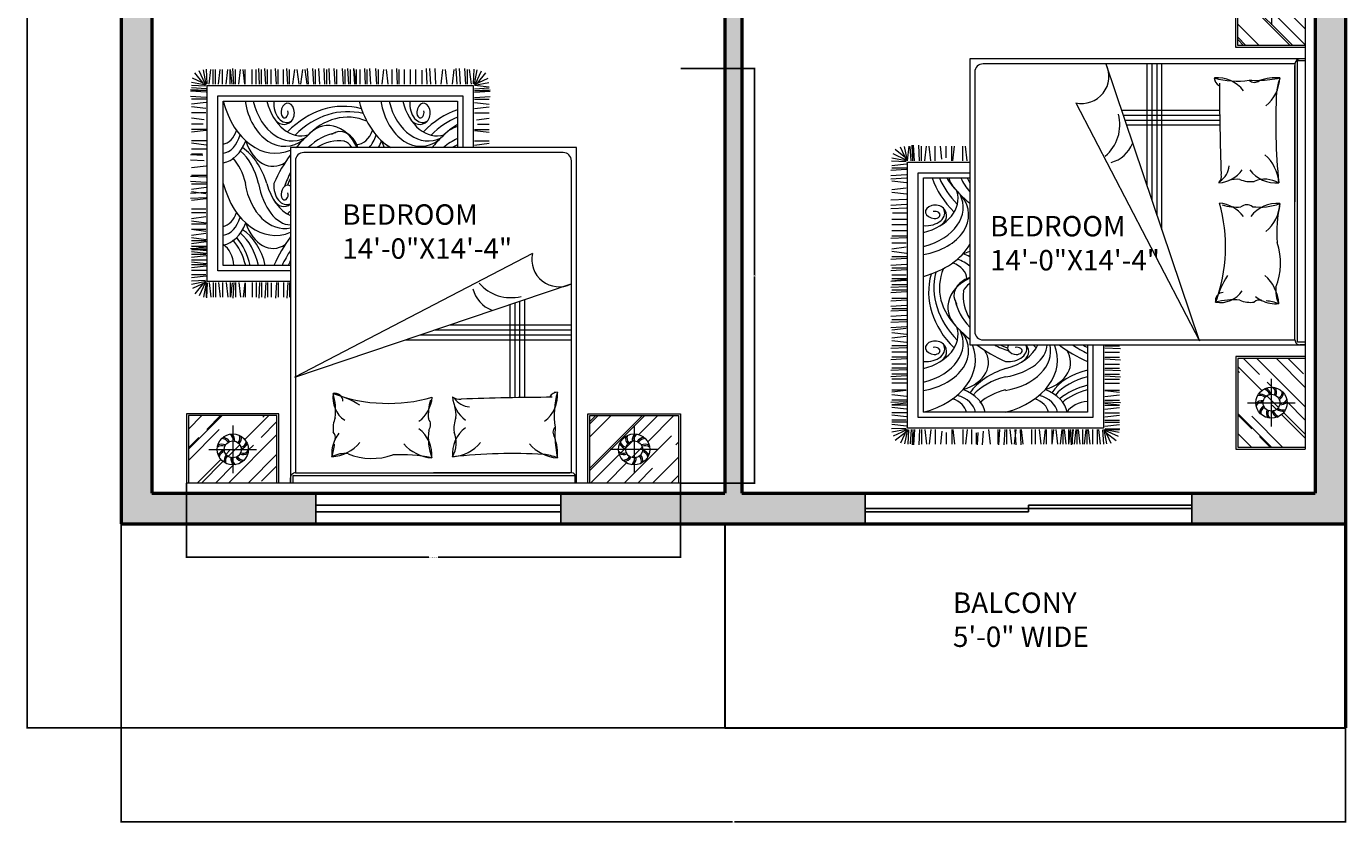
# Model space of a CAD drawing. Units: inches. Extents: x 2831 to 3729, y 3926 to 4974.
# Tile 5 of 8: x 3313 to 3701, y 4438 to 4672. Entities that reach past the tile are written whole.
import ezdxf

# ---------------------------------------------------------------- set-up
doc = ezdxf.new("R2010")
doc.units = ezdxf.units.IN
for name, color, linetype, lineweight in [('A-ANNO-DIMS', 2, 'Continuous', 18), ('A-AREA-IDEN', 7, 'Continuous', 18), ('A-DOOR', 3, 'Continuous', 25), ('A-FLOR', 7, 'Continuous', 30), ('A-FURN', 8, 'Continuous', 18), ('A-GLAZ', 4, 'Continuous', 25), ('A-WALL', 7, 'Continuous', 50), ('A-WALL-PATT', 252, 'Continuous', 13)]:
    doc.layers.add(name, color=color, linetype=linetype, lineweight=lineweight)
doc.styles.get("Standard").update_dxf_attribs({"font": 'arial.ttf'})
doc.dimstyles.get("Standard").update_dxf_attribs({"dimtxt": 0.18, "dimasz": 0.18, "dimexe": 0.18, "dimexo": 0.0625, "dimgap": 0.09, "dimtad": 0, "dimtih": 1, "dimtoh": 1, "dimdec": 4, "dimzin": 0, "dimdsep": 46, "dimtxsty": 'Standard', "dimcen": 0.09, "dimadec": 0, "dimazin": 0, "dimtfac": 1, "dimtdec": 4, "dimtofl": 0, "dimtmove": 0, "dimatfit": 3, "dimfxl": 1, "dimtolj": 1, "dimtzin": 0, "dimarcsym": 0})

# ---------------------------------------------------------------- blocks, each defined once
blk = doc.blocks.new('A$C64B41DC1')
for p, q in [((0, 2.5079), (2.9903, 2.5079)), ((0, 2.0879), (0, 2.5079)), ((0.012, 2.4618), (0.0581, 2.5079)), ((0.012, 2.3515), (0.1684, 2.5079)), ((0.012, 2.0999), (0.012, 2.5079)), ((0.0543, 2.2213), (0.3409, 2.5079)), ((0.1689, 2.4179), (0.2589, 2.5079)), ((0.3265, 2.386), (0.4484, 2.5079)), ((0.3699, 2.3332), (0.5445, 2.5079)), ((0.548, 2.5079), (0.548, 2.0999)), ((0.56, 2.5079), (0.56, 2.0879)), ((0.6301, 2.5079), (0.6301, 0.4779)), ((0.6401, 2.461), (0.6401, 2.5079)), ((0.6401, 2.5079), (2.344, 2.5079)), ((2.344, 2.5079), (2.3601, 2.5079)), ((2.344, 2.5079), (2.344, 2.461)), ((2.3601, 2.5079), (2.3601, 2.4761)), ((2.3601, 0.4779), (2.3601, 2.5079)), ((2.4303, 2.5079), (2.4303, 2.0879)), ((2.4423, 2.5079), (2.4423, 2.0999)), ((2.4423, 2.3333), (2.6169, 2.5079)), ((2.4423, 2.2145), (2.7357, 2.5079)), ((2.4423, 2.404), (2.5354, 2.4971)), ((2.705, 2.398), (2.8149, 2.5079)), ((2.7691, 2.3772), (2.8998, 2.5079)), ((2.7819, 2.3646), (2.9252, 2.5079)), ((2.9783, 2.0999), (2.9783, 2.5079)), ((2.9903, 2.0879), (2.9903, 2.5079)), ((0.2157, 2.0999), (0.548, 2.4322)), ((0.2299, 2.0999), (0.548, 2.418)), ((0.2804, 2.1597), (0.2804, 2.4481)), ((2.344, 2.461), (0.6401, 2.461)), ((0.6601, 2.4461), (1.4951, 2.4461)), ((0.6601, 2.4461), (0.6601, 0.5579)), ((1.4951, 2.4461), (0.6697, 2.4461)), ((2.3301, 2.4461), (1.4951, 2.4461)), ((2.3301, 0.5579), (2.3301, 2.4461)), ((2.7099, 2.1597), (2.7099, 2.4481)), ((0.2311, 2.2906), (0.2937, 2.3532)), ((0.3405, 2.3039), (0.3605, 2.3238)), ((2.6158, 2.3088), (2.6313, 2.3243)), ((2.6674, 2.2756), (2.7382, 2.3464)), ((2.7249, 2.3076), (2.7512, 2.3339)), ((2.7914, 2.1846), (2.9783, 2.3715)), ((0.012, 2.261), (0.0275, 2.2765)), ((0.0404, 2.0999), (0.1982, 2.2578)), ((0.1362, 2.3039), (0.4246, 2.3039)), ((0.2905, 2.2539), (0.3304, 2.2938)), ((2.4918, 2.0999), (2.6366, 2.2447)), ((2.8541, 2.3039), (2.5657, 2.3039)), ((2.5849, 2.2779), (2.6158, 2.3088)), ((2.7746, 2.0999), (2.9783, 2.3036)), ((2.9144, 2.2312), (2.9783, 2.2951)), ((0.1365, 2.0999), (0.251, 2.2144)), ((0.4194, 2.0999), (0.548, 2.2285)), ((2.4423, 2.1353), (2.5382, 2.2312)), ((2.7831, 2.0999), (2.8678, 2.1846)), ((2.8962, 2.0999), (2.9783, 2.182)), ((0.56, 2.0879), (0, 2.0879)), ((0.548, 2.0999), (0.012, 2.0999)), ((0.4986, 2.0999), (0.548, 2.1493)), ((0.5127, 2.0999), (0.548, 2.1352)), ((2.4303, 2.0879), (2.9903, 2.0879)), ((2.4423, 2.0999), (2.9783, 2.0999)), ((2.5172, 2.0999), (2.5269, 2.1096)), ((0.9415, 1.9902), (0.9415, 1.3975)), ((0.9715, 1.9906), (0.9715, 1.4076)), ((1.0015, 1.991), (1.0015, 1.4177)), ((1.0315, 1.9916), (1.0315, 1.4279)), ((2.3349, 1.8678), (0.6613, 1.3029)), ((0.8956, 1.1191), (2.3349, 1.8678)), ((1.6636, 1.6412), (0.6601, 1.6412)), ((1.5748, 1.6112), (0.6601, 1.6112)), ((2.3665, 1.295), (2.3665, 1.3839)), ((2.377, 1.295), (2.3822, 1.3891)), ((2.4032, 1.295), (2.4032, 1.3839)), ((2.4346, 1.295), (2.4346, 1.3839)), ((2.4451, 1.295), (2.4503, 1.3891)), ((2.4774, 1.2957), (2.4774, 1.3837)), ((2.5, 1.295), (2.5, 1.3839)), ((2.5105, 1.295), (2.5157, 1.3891)), ((2.5367, 1.295), (2.5367, 1.3839)), ((2.5471, 1.295), (2.5524, 1.3891)), ((2.5681, 1.295), (2.5681, 1.3839)), ((2.5918, 1.295), (2.5918, 1.3839)), ((2.6346, 1.2957), (2.6346, 1.3837)), ((2.6362, 1.2957), (2.6467, 1.3839)), ((2.6729, 1.295), (2.6624, 1.3839)), ((2.6938, 1.295), (2.6938, 1.3839)), ((2.7043, 1.295), (2.7095, 1.3891)), ((2.7127, 1.2957), (2.7232, 1.3839)), ((2.7253, 1.295), (2.7253, 1.3839)), ((2.7494, 1.295), (2.7389, 1.3839)), ((2.7718, 1.295), (2.7718, 1.3839)), ((2.7959, 1.295), (2.7854, 1.3839)), ((2.8146, 1.2957), (2.8146, 1.3837)), ((2.8146, 1.2957), (2.8146, 1.3837)), ((2.8282, 1.295), (2.8282, 1.3839)), ((2.8282, 1.295), (2.8282, 1.3839)), ((2.8523, 1.295), (2.8418, 1.3839)), ((2.8523, 1.295), (2.8418, 1.3839)), ((2.8653, 1.2966), (2.8688, 1.3861)), ((2.8711, 1.2957), (2.8711, 1.3837)), ((2.8711, 1.2957), (2.8875, 1.3822)), ((2.8765, 1.2958), (2.9132, 1.3758)), ((2.8893, 1.3011), (2.9394, 1.3636)), ((2.3601, 1.2873), (2.8639, 1.2873)), ((2.8639, 1.2873), (2.8639, 0.1018)), ((2.8713, 1.2927), (2.954, 1.3315)), ((2.8717, 1.2884), (2.9588, 1.3058)), ((2.8744, 1.2817), (2.9603, 1.2869)), ((2.3601, 1.2233), (2.7999, 1.2233)), ((2.7999, 1.2233), (2.7999, 0.1658)), ((2.8716, 1.2565), (2.9605, 1.2669)), ((2.8716, 1.2212), (2.9605, 1.2212)), ((2.8716, 1.1947), (2.9605, 1.2052)), ((2.8723, 1.2489), (2.9603, 1.2489)), ((2.3601, 1.1913), (2.7679, 1.1912)), ((2.7679, 1.1912), (2.7679, 0.1978)), ((2.8716, 1.181), (2.9605, 1.1705)), ((2.8716, 1.1595), (2.9605, 1.1595)), ((2.8716, 1.133), (2.9605, 1.1435)), ((2.8716, 1.1193), (2.9605, 1.1088)), ((2.8723, 1.1872), (2.9603, 1.1872)), ((2.8723, 1.1255), (2.9603, 1.1255)), ((2.8716, 1.1035), (2.9605, 1.093)), ((2.8716, 1.0965), (2.9605, 1.0965)), ((2.8716, 1.086), (2.9657, 1.0913)), ((2.8716, 1.0756), (2.9605, 1.0756)), ((2.8716, 1.0491), (2.9605, 1.0596)), ((2.8723, 1.0858), (2.9605, 1.0753)), ((2.8723, 1.0416), (2.9603, 1.0416)), ((2.8716, 1.0354), (2.9605, 1.0249)), ((2.8723, 0.9987), (2.9605, 1.0092)), ((2.8723, 0.985), (2.9605, 0.9745)), ((2.8723, 0.9735), (2.9603, 0.9735)), ((2.8716, 0.9346), (2.9605, 0.9241)), ((2.8723, 0.9408), (2.9603, 0.9408)), ((2.8723, 0.8979), (2.9605, 0.9084)), ((2.8716, 0.7885), (2.9605, 0.799)), ((2.8723, 0.8726), (2.9603, 0.8726)), ((2.8723, 0.8505), (2.9603, 0.8505)), ((2.8716, 0.7818), (2.9657, 0.787)), ((2.8716, 0.7503), (2.9657, 0.7556)), ((2.8716, 0.7204), (2.9605, 0.7309)), ((2.8723, 0.7571), (2.9605, 0.7466)), ((2.8716, 0.6995), (2.9605, 0.6995)), ((2.8716, 0.689), (2.9657, 0.6838)), ((2.8716, 0.6576), (2.9657, 0.6523)), ((2.8716, 0.6471), (2.9605, 0.6471)), ((2.8716, 0.5903), (2.9605, 0.6007)), ((0.7101, 0.5079), (2.2801, 0.5079)), ((2.8716, 0.4877), (2.9603, 0.4877)), ((2.882, 0.5582), (2.9657, 0.5536)), ((2.8909, 0.5263), (2.9657, 0.5222)), ((2.8928, 0.5169), (2.9605, 0.5169)), ((0.6301, 0.4779), (2.3601, 0.4779)), ((1.2465, 0.4625), (1.1576, 0.452)), ((1.2465, 0.4365), (1.1577, 0.4365)), ((1.2542, 0.1018), (1.2542, 0.4779)), ((1.3182, 0.1658), (1.3182, 0.4779)), ((1.3502, 0.1978), (1.3502, 0.4779)), ((2.8716, 0.4625), (2.9605, 0.452)), ((2.8716, 0.4365), (2.9603, 0.4365)), ((1.2465, 0.3746), (1.1576, 0.3851)), ((1.2465, 0.3684), (1.1577, 0.3684)), ((1.2285, 0.3357), (1.1577, 0.3357)), ((2.8716, 0.3746), (2.9605, 0.3851)), ((2.8716, 0.3684), (2.9603, 0.3684)), ((2.8896, 0.3357), (2.9603, 0.3357)), ((1.2355, 0.3092), (1.1576, 0.3)), ((1.2457, 0.2423), (1.1576, 0.2319)), ((1.2457, 0.2676), (1.1577, 0.2676)), ((2.8723, 0.2676), (2.9603, 0.2676)), ((2.8723, 0.2423), (2.9605, 0.2319)), ((2.8826, 0.3092), (2.9605, 0.3)), ((1.2465, 0.1742), (1.1524, 0.169)), ((1.2465, 0.2057), (1.1576, 0.2161)), ((1.2465, 0.1847), (1.1576, 0.1847)), ((2.7999, 0.1658), (1.3182, 0.1658)), ((2.7679, 0.1978), (1.3502, 0.1978)), ((2.8716, 0.2057), (2.9605, 0.2161)), ((2.8716, 0.1847), (2.9605, 0.1847)), ((2.8716, 0.1742), (2.9657, 0.169)), ((1.2465, 0.1428), (1.1524, 0.1376)), ((1.2465, 0.1334), (1.1524, 0.1281)), ((1.2465, 0.1323), (1.1576, 0.1323)), ((1.2465, 0.1323), (1.1576, 0.1323)), ((1.2465, 0.1), (1.1576, 0.1105)), ((1.2465, 0.1229), (1.1588, 0.1168)), ((1.2464, 0.1007), (1.1592, 0.0833)), ((1.2468, 0.0964), (1.1641, 0.0576)), ((1.2288, 0.088), (1.1787, 0.0255)), ((1.2415, 0.0933), (1.2049, 0.0133)), ((1.247, 0.0934), (1.2306, 0.0069)), ((1.2527, 0.0925), (1.2493, 0.003)), ((2.8639, 0.1018), (1.2542, 0.1018)), ((1.2658, 0.0941), (1.2762, 0.0052)), ((1.2899, 0.0941), (1.2899, 0.0052)), ((1.2999, 0.0941), (1.3051, 0)), ((1.3313, 0.0941), (1.3365, 0)), ((1.3523, 0.0941), (1.3575, 0)), ((1.3804, 0.0941), (1.3699, 0.0052)), ((1.4119, 0.0934), (1.4223, 0.0052)), ((1.4485, 0.0941), (1.438, 0.0052)), ((1.48, 0.0941), (1.4852, 0)), ((1.5114, 0.0941), (1.5166, 0)), ((1.5323, 0.0941), (1.5376, 0)), ((1.5638, 0.0941), (1.5638, 0.0105)), ((1.6021, 0.0941), (1.6021, 0.0052)), ((1.6336, 0.0941), (1.6336, 0.0052)), ((1.6702, 0.0941), (1.6702, 0.0052)), ((1.7017, 0.0941), (1.7017, 0.0052)), ((1.7122, 0.0941), (1.7174, 0)), ((1.7445, 0.0934), (1.7445, 0.0054)), ((1.7698, 0.0934), (1.7803, 0.0052)), ((1.8065, 0.0941), (1.796, 0.0052)), ((1.8274, 0.0941), (1.8274, 0.0052)), ((1.8379, 0.0941), (1.8431, 0)), ((1.8746, 0.0941), (1.8798, 0)), ((1.8955, 0.0941), (1.8955, 0.0052)), ((1.906, 0.0941), (1.9113, 0)), ((1.9384, 0.0934), (1.9384, 0.0054)), ((1.9609, 0.0941), (1.9609, 0.0052)), ((1.9636, 0.0934), (1.9741, 0.0052)), ((1.9714, 0.0941), (1.9766, 0)), ((1.9976, 0.0941), (1.9976, 0.0052)), ((2.0081, 0.0941), (2.0133, 0)), ((2.029, 0.0941), (2.029, 0.0052)), ((2.0395, 0.0941), (2.0447, 0)), ((2.0797, 0.0941), (2.0797, 0.0052)), ((2.0902, 0.0941), (2.0954, 0)), ((2.1216, 0.0941), (2.1269, 0)), ((2.1412, 0.0941), (2.1412, 0.0052)), ((2.1517, 0.0941), (2.1569, 0)), ((2.1831, 0.0941), (2.1884, 0)), ((2.2093, 0.0941), (2.2093, 0.0052)), ((2.2198, 0.0941), (2.225, 0)), ((2.2512, 0.0941), (2.2565, 0)), ((2.2603, 0.0934), (2.2707, 0.0052)), ((2.2969, 0.0941), (2.2864, 0.0052)), ((2.3089, 0.0934), (2.3193, 0.0052)), ((2.3455, 0.0941), (2.3351, 0.0052)), ((2.3665, 0.0941), (2.3665, 0.0052)), ((2.377, 0.0941), (2.3822, 0)), ((2.4032, 0.0941), (2.4032, 0.0052)), ((2.4346, 0.0941), (2.4346, 0.0052)), ((2.4451, 0.0941), (2.4503, 0)), ((2.4774, 0.0934), (2.4774, 0.0054)), ((2.5, 0.0941), (2.5, 0.0052)), ((2.5105, 0.0941), (2.5157, 0)), ((2.5367, 0.0941), (2.5367, 0.0052)), ((2.5471, 0.0941), (2.5524, 0)), ((2.5681, 0.0941), (2.5681, 0.0052)), ((2.5918, 0.0941), (2.5918, 0.0052)), ((2.6346, 0.0934), (2.6346, 0.0054)), ((2.6362, 0.0934), (2.6467, 0.0052)), ((2.6729, 0.0941), (2.6624, 0.0052)), ((2.6938, 0.0941), (2.6938, 0.0052)), ((2.7043, 0.0941), (2.7095, 0)), ((2.7127, 0.0934), (2.7232, 0.0052)), ((2.7253, 0.0941), (2.7253, 0.0052)), ((2.7494, 0.0941), (2.7389, 0.0052)), ((2.7718, 0.0941), (2.7718, 0.0052)), ((2.7959, 0.0941), (2.7854, 0.0052)), ((2.8146, 0.0934), (2.8146, 0.0054)), ((2.8282, 0.0941), (2.8282, 0.0052)), ((2.8523, 0.0941), (2.8418, 0.0052)), ((2.8653, 0.0925), (2.8688, 0.003)), ((2.8711, 0.0934), (2.8875, 0.0069)), ((2.8713, 0.0964), (2.954, 0.0576)), ((2.8716, 0.1428), (2.9657, 0.1376)), ((2.8716, 0.1334), (2.9657, 0.1281)), ((2.8716, 0.1323), (2.9605, 0.1323)), ((2.8716, 0.1229), (2.9593, 0.1168)), ((2.8717, 0.1007), (2.9588, 0.0833)), ((2.8744, 0.1074), (2.9603, 0.1022)), ((2.8765, 0.0933), (2.9132, 0.0133)), ((2.8893, 0.088), (2.9394, 0.0255))]:
    blk.add_line(p, q)
at = {"ltscale": 10}
for p, q in [((1.4859, 1.5812), (0.6601, 1.5812)), ((1.397, 1.5512), (0.6601, 1.5512))]:
    blk.add_line(p, q, dxfattribs=at)
for centre, radius in [((0.2804, 2.3039), 0.0942), ((2.7099, 2.3039), 0.0942), ((0.2804, 2.3039), 0.051), ((2.7099, 2.3039), 0.051)]:
    blk.add_circle(centre, radius)
for centre, radius, start, end in [((0.6601, 2.4761), 0.03, 180, 270), ((2.3301, 2.4761), 0.03, 270, 0), ((0.3286, 2.3561), 0.0605, 136.17003, 182.48975), ((0.3231, 2.3585), 0.0462, 124.30017, 184.53802), ((2.6672, 2.3585), 0.0462, 355.46198, 55.69983), ((2.6617, 2.3561), 0.0605, 357.51025, 43.82997), ((0.2457, 2.3659), 0.0605, 208.17003, 254.48975), ((0.2417, 2.3614), 0.0462, 196.30017, 256.53802), ((0.2887, 2.3745), 0.0605, 172.17003, 218.48975), ((0.2828, 2.3731), 0.0462, 160.30017, 220.53802), ((0.3501, 2.3178), 0.0605, 100.17003, 146.48975), ((0.347, 2.323), 0.0462, 88.30017, 148.53802), ((0.3449, 2.2742), 0.0605, 64.17003, 110.48975), ((0.3455, 2.2802), 0.0462, 52.30017, 112.53802), ((1.0526, 2.3302), 0.3085, 175.30484, 198.69419), ((-0.8702, 2.0941), 1.6364, 4.80985, 9.18918), ((0.8579, 2.6278), 0.2948, 247.51785, 264.26696), ((0.728, 2.111), 0.245, 40.4189, 85.9871), ((1.0164, 5.7096), 3.3803, 266.81337, 276.16021), ((1.3963, 2.1044), 0.245, 94.0129, 139.5811), ((1.1858, 2.3288), 0.1943, 306.5711, 5.88998), ((1.5348, 2.2652), 0.1767, 151.77364, 201.69827), ((1.6986, 2.3355), 0.1943, 174.11002, 233.4289), ((1.1481, 2.2311), 0.3783, 353.49469, 19.18669), ((1.6871, 3.192), 0.8561, 257.74383, 273.62843), ((1.4882, 2.111), 0.245, 40.4189, 85.9871), ((1.8674, 1.9709), 0.3878, 68.20259, 108.9817), ((2.1269, 2.1044), 0.245, 94.0129, 139.5811), ((2.0342, 2.4856), 0.1563, 261.59582, 298.90918), ((1.9165, 2.3288), 0.1943, 333.73715, 5.88998), ((2.6058, 2.2028), 0.517, 163.60457, 172.3273), ((2.6448, 2.2802), 0.0462, 67.46198, 127.69983), ((2.6454, 2.2742), 0.0605, 69.51025, 115.82997), ((2.6433, 2.323), 0.0462, 31.46198, 91.69983), ((2.6402, 2.3178), 0.0605, 33.51025, 79.82997), ((2.7075, 2.3731), 0.0462, 319.46198, 19.69983), ((2.7016, 2.3745), 0.0605, 321.51025, 7.82997), ((2.7486, 2.3614), 0.0462, 283.46198, 343.69983), ((2.7446, 2.3659), 0.0605, 285.51025, 331.82997), ((0.2153, 2.3276), 0.0462, 232.30017, 292.53802), ((0.2158, 2.3336), 0.0605, 244.17003, 290.48975), ((0.2138, 2.2848), 0.0462, 268.30017, 328.53802), ((0.2107, 2.29), 0.0605, 280.17003, 326.48975), ((0.2377, 2.2493), 0.0462, 304.30017, 4.53802), ((0.2322, 2.2517), 0.0605, 316.17003, 2.48975), ((0.2779, 2.2347), 0.0462, 340.30017, 40.53802), ((0.272, 2.2333), 0.0605, 352.17003, 38.48975), ((0.3191, 2.2464), 0.0462, 16.30017, 76.53802), ((0.3151, 2.2419), 0.0605, 28.17003, 74.48975), ((1.9165, 2.3288), 0.1943, 320.94042, 333.73715), ((2.1347, 2.2313), 0.0459, 165.35061, 223.26844), ((2.6752, 2.2419), 0.0605, 105.51025, 151.82997), ((2.6712, 2.2464), 0.0462, 103.46198, 163.69983), ((2.7182, 2.2333), 0.0605, 141.51025, 187.82997), ((2.7123, 2.2347), 0.0462, 139.46198, 199.69983), ((2.7581, 2.2517), 0.0605, 177.51025, 223.82997), ((2.7526, 2.2493), 0.0462, 175.46198, 235.69983), ((2.7796, 2.29), 0.0605, 213.51025, 259.82997), ((2.7765, 2.2848), 0.0462, 211.46198, 271.69983), ((2.7744, 2.3336), 0.0605, 249.51025, 295.82997), ((2.775, 2.3276), 0.0462, 247.46198, 307.69983), ((0.2688, 2.0945), 0.4956, 344.0243, 8.70709), ((0.7274, 2.2013), 0.0446, 314.4736, 42.17134), ((-1.6008, 2.277), 2.3618, 357.39054, 358.88764), ((1.204, 2.1778), 0.1681, 337.01697, 7.53676), ((1.5671, 2.1546), 0.0547, 142.08329, 220.902), ((1.9346, 2.1778), 0.1681, 337.01697, 7.53676), ((0.9385, 1.978), 0.1943, 126.5711, 185.88998), ((1.1858, 1.9714), 0.1943, 4.31813, 53.4289), ((1.5415, 2.0969), 0.1834, 175.22328, 196.23004), ((1.7059, 1.9714), 0.204, 127.11975, 175.09005), ((1.1965, 2.0983), 0.3299, 343.79543, 3.55541), ((1.9394, 1.991), 0.1651, 351.26213, 55.75721), ((2.4617, 2.0719), 0.3745, 173.82958, 196.4356), ((0.7246, 18.8439), 16.8552, 270.17399, 272.05214), ((1.2687, 1.9248), 0.1223, 33.62799, 86.47438), ((1.3401, 1.9404), 0.0603, 49.09906, 101.37023), ((1.7676, 1.0629), 0.9631, 69.65065, 105.96307), ((2.2748, 2.5795), 0.6373, 238.34989, 254.31375), ((2.0911, 2.0123), 0.0478, 179.77267, 283.80184), ((0.7417, 2.0149), 0.057, 273.47085, 328.54118), ((0.728, 2.2025), 0.245, 274.0129, 278.34166), ((1.0747, 1.2871), 0.1871, 14.1863, 69.12121), ((1.0274, 1.1334), 0.2527, 40.62904, 104.37123), ((0.7347, 1.1553), 0.1649, 347.31088, 116.44537), ((0.7101, 0.5579), 0.05, 180, 270), ((2.2801, 0.5579), 0.05, 270, 0)]:
    blk.add_arc(centre, radius, start, end)
for centre, major_axis, ratio, start_param, end_param in [((1.9938, 1.6262), (0, -0.7531), 0.68, 0.797284, 0.954936), ((2.0643, 1.466), (0, -0.5322), 0.68, 7.239912, 7.311536), ((1.9052, 1.7397), (0, -0.9842), 0.68, 0.74745, 0.979724), ((2.4665, 0.8216), (0, -0.2664), 0.68, 2.006169, 3.565187), ((2.7455, 1.3081), (0, 0.3614), 0.68, 1.900046, 2.742661), ((2.7868, 1.3081), (0, 0.3614), 0.68, 1.900046, 2.614747), ((2.8372, 1.3081), (0, 0.3614), 0.68, 1.900046, 2.479658), ((2.8607, 1.3211), (0, 0.3614), 0.68, 1.938265, 2.479658), ((2.8057, 1.2079), (0, -0.1524), 0.68, 4.821745, 5.895886), ((2.4513, 0.5069), (0, 0.502), 0.68, 5.095327, 6.553458), ((2.7862, 0.8069), (0, -0.2615), 0.68, 3.244645, 4.205018), ((2.396, 0.6032), (0, 0.3641), 0.68, -1.3172, 0.145284), ((2.7784, 0.8289), (0, -0.1802), 0.68, 3.227058, 4.318474), ((2.3507, 0.5642), (0.0073, 0.3819), 0.56205, -1.21172, -0.009991), ((2.2964, 0.5771), (0, -0.3263), 0.68, 1.938944, 2.850232), ((2.0403, 1.6015), (0, -0.8763), 0.68, 6.849801, 6.887077), ((2.7821, 0.7971), (0, -0.1589), 0.68, 3.272942, 4.229533), ((2.4005, 0.7132), (0, -0.1214), 0.68, 2.284368, 3.652258), ((2.3834, 0.7081), (0, 0.1147), 0.68, 4.593909, 6.585576), ((2.3774, 0.7653), (0, -0.0593), 0.68, 5.841311, 7.755362), ((2.3961, 0.7628), (0, -0.0317), 0.68, 1.462497, 5.046281), ((1.9938, 1.1295), (-0.0678, 0.7439), 0.610498, 3.917146, 4.063997), ((2.0643, 0.9693), (0, -0.5322), 0.68, 7.239912, 7.336618), ((1.9052, 1.243), (0, -0.9842), 0.68, 0.74745, 0.979724), ((2.7455, 0.8114), (-0.0599, 0.3735), 0.695517, 1.775813, 2.548612), ((2.7868, 0.8114), (0, 0.3614), 0.68, 1.900046, 2.614747), ((2.8607, 0.8243), (0, 0.3614), 0.68, 1.938265, 2.479658), ((2.4513, 0.0102), (0, 0.502), 0.68, 5.095327, 6.553458), ((2.4665, 0.3249), (0, -0.2664), 0.68, 2.006169, 3.565187), ((2.7862, 0.3102), (0, -0.2615), 0.68, 3.244645, 4.205018), ((1.5283, 0.0674), (0, -0.3703), 0.68, 1.930561, 3.464283), ((1.5736, 0.1065), (0, 0.3641), 0.68, -1.3172, 0.476403), ((2.3507, 0.0674), (0, -0.3703), 0.68, 1.930561, 3.464283), ((2.396, 0.1065), (0, 0.3641), 0.68, -1.3172, 0.476403), ((2.7784, 0.3322), (0, -0.1802), 0.68, 3.227058, 4.318474), ((1.242, 0.9693), (0, -0.5322), 0.68, 6.586764, 6.677612), ((1.1714, 1.1295), (-0.1157, 0.7241), 0.59432, 3.291697, 3.50733), ((1.1933, 0.9181), (0, -0.624), 0.68, 0.378672, 0.625379), ((1.3091, 0.6603), (0, -0.3155), 0.68, 6.475719, 6.949396), ((1.1911, 1.1066), (0, 0.8458), 0.68, 3.421828, 3.728616), ((1.474, 0.0804), (0, -0.3263), 0.68, 1.938944, 3.339184), ((1.0828, 1.243), (0, -0.9842), 0.68, 0.565948, 0.680366), ((1.6289, 0.0102), (0, 0.502), 0.68, 6.655152, 6.661293), ((1.6289, 0.0102), (0, 0.502), 0.68, 5.095327, 5.911219), ((1.6442, 0.3249), (0, -0.2664), 0.68, 2.006169, 2.182797), ((1.9638, 0.3102), (0, -0.2615), 0.68, 4.015924, 4.205018), ((1.956, 0.3322), (0, -0.1802), 0.68, 3.770744, 4.318474), ((1.9597, 0.3004), (0, -0.1589), 0.68, 3.14258, 4.229533), ((2.0157, 0.9181), (0, -0.624), 0.68, -0.280078, 0.625379), ((2.0135, 1.1066), (0, 0.8458), 0.68, 2.978727, 3.728616), ((2.0606, 0.5616), (0, -0.1803), 0.68, 5.194792, 5.929328), ((2.0606, 0.5616), (0, -0.1803), 0.68, 5.194792, 6.723255), ((2.1315, 0.6603), (0, -0.3155), 0.68, 5.328638, 6.949396), ((2.0549, 0.5656), (0, -0.1303), 0.68, 5.450951, 6.054641), ((2.0643, 0.9693), (0, -0.5322), 0.68, 6.20013, 6.677612), ((1.9938, 1.1295), (-0.0678, 0.7439), 0.610498, 3.199135, 3.592282), ((2.2964, 0.0804), (0, -0.3263), 0.68, 1.938944, 3.339184), ((1.9052, 1.243), (0, -0.9842), 0.68, 0.565948, 0.680366), ((2.4513, 0.0102), (0, 0.502), 0.68, 6.655152, 6.661293), ((2.7821, 0.3004), (0, -0.1589), 0.68, 3.272942, 4.229533), ((1.2179, 1.1047), (0, -0.8763), 0.68, 6.507006, 6.887077), ((1.5781, 0.2165), (0, -0.1214), 0.68, 2.284368, 3.726131), ((1.561, 0.2114), (0, 0.1147), 0.68, 4.593909, 6.647252), ((2.0403, 1.1047), (0, -0.8763), 0.68, 6.099302, 6.887077), ((2.4005, 0.2165), (0, -0.1214), 0.68, 2.284368, 3.726131), ((2.3834, 0.2114), (0, 0.1147), 0.68, 4.593909, 6.647252), ((1.555, 0.2685), (0, -0.0593), 0.68, 3.732151, 7.755362), ((1.5737, 0.2661), (0, -0.0317), 0.68, 1.462497, 5.046281), ((2.3774, 0.2685), (0, -0.0593), 0.68, 3.732151, 7.755362), ((2.3961, 0.2661), (0, -0.0317), 0.68, 1.462497, 5.046281)]:
    blk.add_ellipse(centre, major_axis=major_axis, ratio=ratio, start_param=start_param, end_param=end_param)
blk = doc.blocks.new('WINDOW-72IN-PLAN')
for p, q in [((0, 0), (0, 9)), ((72, 0), (72, 9)), ((72, 5.5), (0, 5.5)), ((72, 3.5), (0, 3.5))]:
    blk.add_line(p, q)
blk = doc.blocks.new('*D33')
at = {"layer": 'A-ANNO-DIMS', "color": 0, "lineweight": -2, "transparency": 16777216}
for p, q in [((3360.51, 4538.01), (3360.51, 4516.11)), ((3505.75, 4538.01), (3505.75, 4516.11)), ((3360.69, 4516.29), (3431.75, 4516.29)), ((3505.57, 4516.29), (3434.51, 4516.29))]:
    blk.add_line(p, q, dxfattribs=at)
at = {"layer": 'A-ANNO-DIMS', "color": 0, "transparency": 16777216}
for points in [[(3360.69, 4516.32), (3360.69, 4516.26), (3360.51, 4516.29)], [(3505.57, 4516.32), (3505.57, 4516.26), (3505.75, 4516.29)]]:
    blk.add_solid(points, dxfattribs=at)
at = {"layer": 'Defpoints', "color": 0, "transparency": 16777216}
for p in [(3360.51, 4538.08), (3505.75, 4538.08), (3360.51, 4516.29)]:
    blk.add_point(p, dxfattribs=at)
at = {"layer": 'A-ANNO-DIMS', "color": 0, "transparency": 16777216, "insert": (3433.13, 4516.29), "char_height": 0.18, "attachment_point": 5}
blk.add_mtext('\\A1;BED GROUP 145 TYP.', dxfattribs=at)
blk = doc.blocks.new('*D34')
at = {"layer": 'A-ANNO-DIMS', "color": 0, "lineweight": -2, "transparency": 16777216}
for p, q in [((3505.82, 4659.89), (3527.72, 4659.89)), ((3527.54, 4659.71), (3527.54, 4599.16)), ((3527.54, 4538.26), (3527.54, 4598.8)), ((3505.82, 4538.08), (3527.72, 4538.08))]:
    blk.add_line(p, q, dxfattribs=at)
at = {"layer": 'A-ANNO-DIMS', "color": 0, "transparency": 16777216}
for points in [[(3527.51, 4659.71), (3527.57, 4659.71), (3527.54, 4659.89)], [(3527.51, 4538.26), (3527.57, 4538.26), (3527.54, 4538.08)]]:
    blk.add_solid(points, dxfattribs=at)
at = {"layer": 'Defpoints', "color": 0, "transparency": 16777216}
for p in [(3505.75, 4659.89), (3505.75, 4538.08), (3527.54, 4538.08)]:
    blk.add_point(p, dxfattribs=at)
at = {"layer": 'A-ANNO-DIMS', "color": 0, "transparency": 16777216, "insert": (3527.54, 4598.98), "char_height": 0.18, "attachment_point": 5}
blk.add_mtext('\\A1;122 TYP.', dxfattribs=at)
blk = doc.blocks.new('*D54')
at = {"layer": 'A-ANNO-DIMS', "color": 0, "lineweight": -2, "transparency": 16777216}
for p, q in [((3341.31, 4526.08), (3341.31, 4438.31)), ((3701.31, 4466.08), (3701.31, 4438.31)), ((3341.49, 4438.49), (3521.02, 4438.49)), ((3701.13, 4438.49), (3521.6, 4438.49))]:
    blk.add_line(p, q, dxfattribs=at)
at = {"layer": 'A-ANNO-DIMS', "color": 0, "transparency": 16777216}
for points in [[(3341.49, 4438.52), (3341.49, 4438.46), (3341.31, 4438.49)], [(3701.13, 4438.52), (3701.13, 4438.46), (3701.31, 4438.49)]]:
    blk.add_solid(points, dxfattribs=at)
at = {"layer": 'Defpoints', "color": 0, "transparency": 16777216}
for p in [(3341.31, 4526.14), (3701.31, 4466.14), (3701.31, 4438.49)]:
    blk.add_point(p, dxfattribs=at)
at = {"layer": 'A-ANNO-DIMS', "color": 0, "transparency": 16777216, "insert": (3521.31, 4438.49), "char_height": 0.18, "attachment_point": 5}
blk.add_mtext('\\A1;360', dxfattribs=at)
blk = doc.blocks.new('*D55')
at = {"layer": 'A-ANNO-DIMS', "color": 0, "lineweight": -2, "transparency": 16777216}
for p, q in [((3341.25, 4946.14), (3313.48, 4946.14)), ((3313.66, 4945.96), (3313.66, 4706.32)), ((3313.66, 4466.32), (3313.66, 4705.96)), ((3518.75, 4466.14), (3313.48, 4466.14))]:
    blk.add_line(p, q, dxfattribs=at)
at = {"layer": 'A-ANNO-DIMS', "color": 0, "transparency": 16777216}
for points in [[(3313.63, 4945.96), (3313.69, 4945.96), (3313.66, 4946.14)], [(3313.63, 4466.32), (3313.69, 4466.32), (3313.66, 4466.14)]]:
    blk.add_solid(points, dxfattribs=at)
at = {"layer": 'Defpoints', "color": 0, "transparency": 16777216}
for p in [(3313.66, 4946.14), (3341.31, 4946.14), (3518.81, 4466.14)]:
    blk.add_point(p, dxfattribs=at)
at = {"layer": 'A-ANNO-DIMS', "color": 0, "transparency": 16777216, "insert": (3313.66, 4706.14), "char_height": 0.18, "attachment_point": 5}
blk.add_mtext('\\A1;480', dxfattribs=at)

msp = doc.modelspace()

# ---------------------------------------------------------------- hatches: boundary and pattern name
at = {"layer": 'A-WALL-PATT'}
h = msp.add_hatch(color=256, dxfattribs=at)
h.dxf.hatch_style = 1
h.paths.add_polyline_path([(3482.8091, 4712.1405), (3350.3091, 4712.1405), (3350.3091, 4788.1405), (3482.8091, 4788.1405), (3482.8091, 4793.1405), (3350.3091, 4793.1405), (3350.3091, 4937.1405), (3398.5591, 4937.1405), (3398.5591, 4946.1405), (3341.3091, 4946.1405), (3341.3091, 4526.1405), (3398.5591, 4526.1405), (3398.5591, 4535.1405), (3350.3091, 4535.1405), (3350.3091, 4707.1405), (3482.8091, 4707.1405)])
h = msp.add_hatch(color=256, dxfattribs=at)
h.dxf.hatch_style = 1
h.paths.add_polyline_path([(3701.3091, 4740.594), (3692.3091, 4740.594), (3692.3091, 4707.1405), (3692.3091, 4535.1405), (3656.0591, 4535.1405), (3656.0591, 4526.1405), (3701.3091, 4526.1405)])
h = msp.add_hatch(color=256, dxfattribs=at)
h.dxf.hatch_style = 1
h.paths.add_polyline_path([(3523.8091, 4712.1405), (3518.8091, 4712.1405), (3518.8091, 4535.1405), (3514.8091, 4535.1405), (3470.5591, 4535.1405), (3470.5591, 4526.1405), (3560.0591, 4526.1405), (3560.0591, 4535.1405), (3523.8091, 4535.1405)])

# ---------------------------------------------------------------- linework, layer by layer
at = {"layer": 'A-DOOR'}
for p, q in [((3560.0591, 4535.1405), (3560.0591, 4526.1405)), ((3656.0591, 4535.1405), (3656.0591, 4526.1405)), ((3656.0591, 4530.6405), (3560.0591, 4530.6405)), ((3656.0591, 4531.6405), (3608.0591, 4531.6405)), ((3608.0591, 4531.6405), (3608.0591, 4529.6405)), ((3608.0591, 4529.6405), (3560.0591, 4529.6405))]:
    msp.add_line(p, q, dxfattribs=at)
at = {"layer": 'A-FLOR'}
for p, q in [((3518.8091, 4526.1405), (3518.8091, 4466.1405)), ((3518.8091, 4466.1405), (3701.3091, 4466.1405))]:
    msp.add_line(p, q, dxfattribs=at)
at = {"layer": 'A-WALL'}
for p, q in [((3341.3091, 4946.1405), (3341.3091, 4526.1405)), ((3701.3091, 4946.1405), (3701.3091, 4466.1405)), ((3518.8091, 4712.1405), (3518.8091, 4535.1405)), ((3523.8091, 4712.1405), (3523.8091, 4535.1405)), ((3350.3091, 4707.1405), (3350.3091, 4535.1405)), ((3692.3091, 4707.1405), (3692.3091, 4535.1405)), ((3350.3091, 4535.1405), (3518.8091, 4535.1405)), ((3514.8091, 4535.1405), (3518.8091, 4535.1405)), ((3523.8091, 4535.1405), (3692.3091, 4535.1405)), ((3341.3091, 4526.1405), (3701.3091, 4526.1405))]:
    msp.add_line(p, q, dxfattribs=at)

# ---------------------------------------------------------------- block references
at = {"layer": 'A-FURN', "xscale": 48.57198025145115, "yscale": 48.57198025145115, "zscale": 48.57198025145115}
for p, rotation in [((3567.6073, 4693.324), 270), ((3505.7533, 4659.8912), 180)]:
    msp.add_blockref('A$C64B41DC1', p, dxfattribs=dict(at, rotation=rotation))
at = {"layer": 'A-GLAZ'}
msp.add_blockref('WINDOW-72IN-PLAN', (3398.5591, 4526.1405), dxfattribs=at)

# ---------------------------------------------------------------- texts
at = {"layer": 'A-AREA-IDEN', "char_height": 6, "attachment_point": 1}
for s, insert in [('BEDROOM \\P14\'-0"X14\'-4"', (3406.3235, 4619.9936)), ('BEDROOM \\P14\'-0"X14\'-4"', (3596.7822, 4616.5784)), ('BALCONY\\P5\'-0" WIDE', (3585.8673, 4505.9314))]:
    msp.add_mtext_dynamic_manual_height_columns(s, width=75.661105, gutter_width=12.5, heights=[0], dxfattribs=dict(at, insert=insert))

# ---------------------------------------------------------------- dimensions: what is measured, and where the dimension line sits
at = {"layer": 'A-ANNO-DIMS'}
dim = msp.add_linear_dim(base=(3313.6591, 4946.1405), p1=(3518.8091, 4466.1405), p2=(3341.3091, 4946.1405), angle=90, dimstyle='Standard', override={"dimdec": 0, "dimlfac": 1, "dimrnd": 0, "dimzin": 0, "dimdsep": 46, "dimlunit": 2}, dxfattribs=at)
dim.commit()
dim.dimension.update_dxf_attribs({"geometry": '*D55', "text_midpoint": (3313.6591, 4706.1405)})
for base, p1, p2, angle, text, picture, middle in [((3527.5399, 4538.0774), (3505.7534, 4659.8912), (3505.7534, 4538.0774), 270, '<> TYP.', '*D34', (3527.5399, 4598.9843)), ((3360.5097, 4516.2908), (3505.7534, 4538.0774), (3360.5097, 4538.0774), 180, 'BED GROUP <> TYP.', '*D33', (3433.1315, 4516.2908))]:
    dim = msp.add_linear_dim(base=base, p1=p1, p2=p2, angle=angle, text=text, dimstyle='Standard', override={"dimdec": 0, "dimlfac": 1, "dimrnd": 0, "dimzin": 0, "dimdsep": 46, "dimlunit": 2}, dxfattribs=at)
    dim.commit()
    dim.dimension.update_dxf_attribs({"geometry": picture, "text_midpoint": middle})
dim = msp.add_linear_dim(base=(3701.3091, 4438.4905), p1=(3341.3091, 4526.1405), p2=(3701.3091, 4466.1405), dimstyle='Standard', override={"dimdec": 0, "dimlfac": 1, "dimrnd": 0, "dimzin": 0, "dimdsep": 46, "dimlunit": 2}, dxfattribs=at)
dim.commit()
dim.dimension.update_dxf_attribs({"geometry": '*D54', "text_midpoint": (3521.3091, 4438.4905)})

doc.saveas('drawing.dxf')
